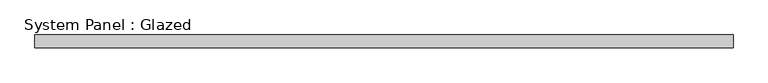
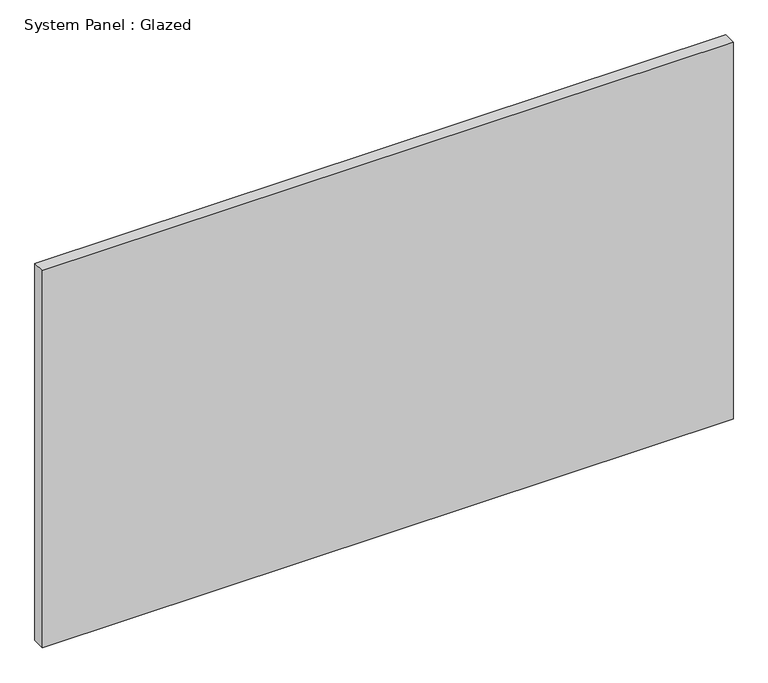
"""IFC4 building model written with IfcOpenShell, lengths in millimetres: plate geometry, System Panel : Glazed."""

from ifc_helpers import new_model, si_unit, origin, origin_with_axes, place, context, project, spatial, polyline, outline, extrude, source, transform, mapped, element, save


def system_panel_glazed_353e56bd(model_context):
    return source(origin(), model_context, "Body", "SweptSolid", [
        extrude(outline(polyline([(692.15, 19.05), (-692.15, 19.05), (-692.15, 44.45), (692.15, 44.45), (692.15, 19.05)])), origin_with_axes(), (0.0, 0.0, 1.0), 798.9054943),
    ])


if __name__ == "__main__":
    model = new_model("IFC4")
    model_context = context("Model", 3, world=origin())
    ifc_project = project(units=[si_unit("LENGTHUNIT", "METRE", prefix="MILLI")], contexts=[model_context])
    site = spatial("IfcSite", under=ifc_project)
    building = spatial("IfcBuilding", under=site)
    placement = place(None, origin())
    system_panel_glazed_shape = system_panel_glazed_353e56bd(model_context)
    element("IfcPlate", 1, ObjectType="System Panel : Glazed", at=placement, inside=building, context=model_context, shape_type="MappedRepresentation", body=[
        mapped(system_panel_glazed_shape, transform((0.0, 0.0, 0.0), x_axis=(1.0, 0.0, 0.0), y_axis=(0.0, 1.0, 0.0), z_axis=(0.0, 0.0, 1.0))),
    ])
    save(model, "model.ifc")

# Revit data of these elements
# Type "System Panel : Glazed"
#   Construction Type Id = "GSP4R"
#   Analytic Construction = "1/8 in Pilkington single glazing"
#   Visual Light Transmittance = 0.9
#   Solar Heat Gain Coefficient = 0.86
#   Heat Transfer Coefficient (U) = 1.18115 BTU/(h·ft²·°F)
#   Define Thermal Properties by = 1
# Element 1 (IfcPlate, "System Panel : Glazed")
#   Materials on its faces: "Glass"
# Materials
#   "Glass": class "Glass", colour RGB 0 128 192, transparency 0.75, Description = "Soda Lime Glass", Cost = 0
